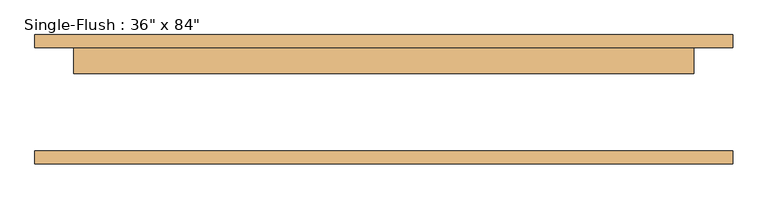
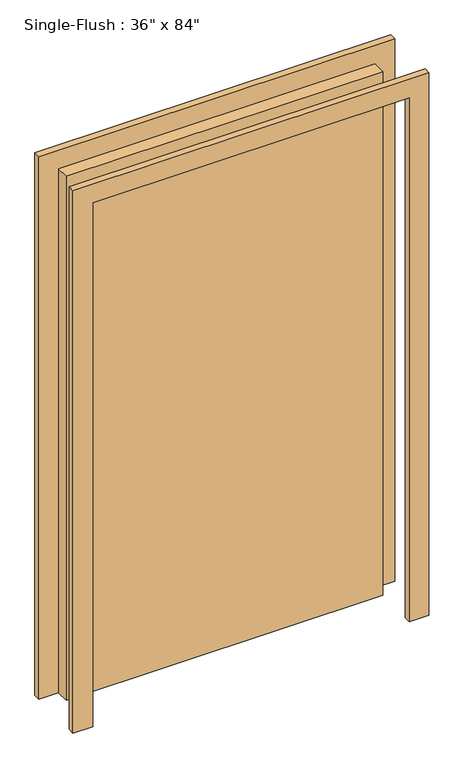
"""IFC4 building model written with IfcOpenShell, lengths in millimetres: door geometry."""

from ifc_helpers import new_model, si_unit, frame, origin, origin_with_axes, place, context, project, spatial, polyline, outline, extrude, source, transform, mapped, element, save


def door_ba16a7d3(model_context):
    return source(origin(), model_context, "Body", "SweptSolid", [
        extrude(outline(polyline([(2209.8, -685.8), (0.0, -685.8), (0.0, -609.6), (2133.6, -609.6), (2133.6, 609.6), (0.0, 609.6), (0.0, 685.8), (2209.8, 685.8), (2209.8, -685.8)])), frame((0.0, 101.6, 0.0), z_axis=(0.0, 1.0, 0.0), x_axis=(0.0, 0.0, 1.0)), (0.0, 0.0, 1.0), 25.4),
        extrude(outline(polyline([(2209.8, 685.8), (2209.8, -685.8), (0.0, -685.8), (0.0, -609.6), (2133.6, -609.6), (2133.6, 609.6), (0.0, 609.6), (0.0, 685.8), (2209.8, 685.8)])), frame((0.0, -127.0, 0.0), z_axis=(0.0, 1.0, 0.0), x_axis=(0.0, 0.0, 1.0)), (0.0, 0.0, 1.0), 25.4),
        extrude(outline(polyline([(609.6, 50.8), (-609.6, 50.8), (-609.6, 101.6), (609.6, 101.6), (609.6, 50.8)])), origin_with_axes(), (0.0, 0.0, 1.0), 2133.6),
    ])


if __name__ == "__main__":
    model = new_model("IFC4")
    model_context = context("Model", 3, world=origin())
    ifc_project = project(units=[si_unit("LENGTHUNIT", "METRE", prefix="MILLI")], contexts=[model_context])
    site = spatial("IfcSite", under=ifc_project)
    building = spatial("IfcBuilding", under=site)
    placement = place(None, origin())
    door_shape = door_ba16a7d3(model_context)
    element("IfcDoor", 1, ObjectType="Single-Flush : 36\" x 84\"", at=placement, inside=building, context=model_context, shape_type="MappedRepresentation", body=[
        mapped(door_shape, transform((0.0, 0.0, 0.0), x_axis=(1.0, 0.0, 0.0), y_axis=(0.0, 1.0, 0.0), z_axis=(0.0, 0.0, 1.0))),
    ])
    save(model, "model.ifc")

# Revit data of these elements
# Type "Single-Flush : 36\" x 84\""
#   Type Mark = "1"
#   Construction Type Id = "MDOOR"
#   Assembly Code = "C1020"
#   Analytic Construction = "Metal"
#   Thickness = 0' - 2"
#   Heat Transfer Coefficient (U) = 0.651978 BTU/(h·ft²·°F)
#   Height = 7' - 0"
#   Trim Projection Ext = 0' - 1"
#   Trim Projection Int = 0' - 1"
#   Trim Width = 0' - 3"
#   Width = 4' - 0"
#   Define Thermal Properties by = 1
#   Door Material = Door - Panel
#   Frame Material = Door - Frame
#   Visual Light Transmittance = 0
#   Solar Heat Gain Coefficient = 0
#   Function = (empty or 0)
#   Wall Closure = (empty or 0)
# Element 1 (IfcDoor, "Single-Flush : 36\" x 84\"")
#   Materials on its faces: "Door - Frame", "Door - Panel"
# Materials
#   "Door - Panel": class "Wood", colour RGB 210 159 95, transparency 0
#   "Door - Frame": colour RGB 118 70 51, transparency 0
